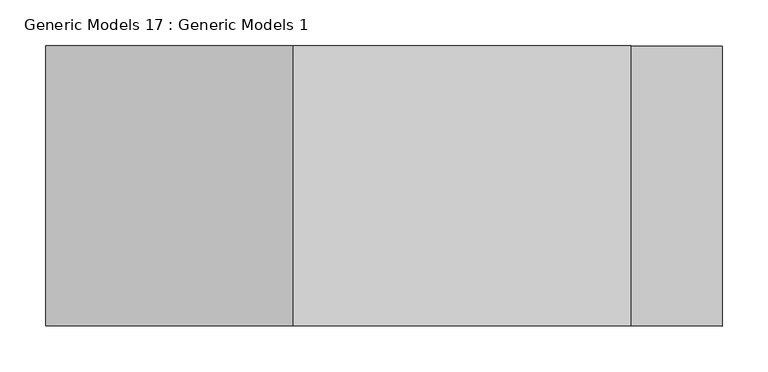
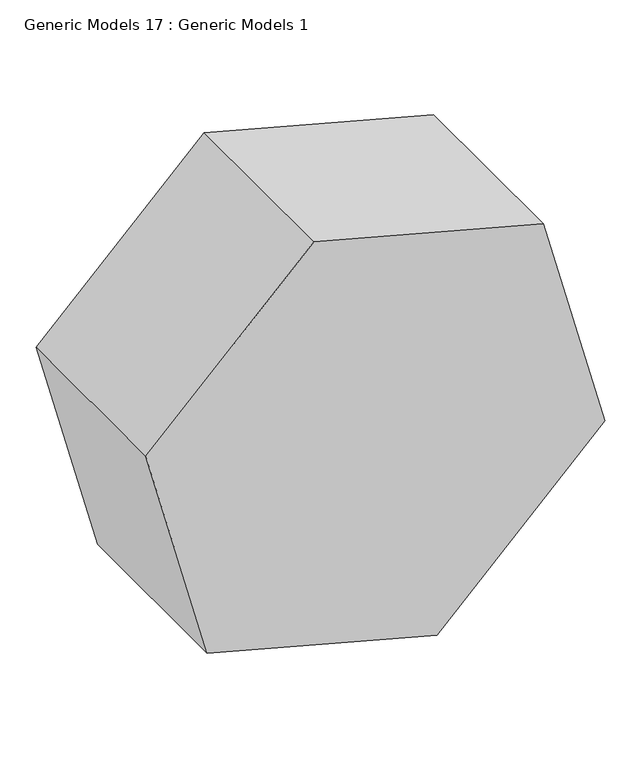
"""IFC4 building model written with IfcOpenShell, lengths in millimetres: proxy geometry, Generic Models 17 : Generic Models 1."""

from ifc_helpers import new_model, si_unit, frame, origin, place, context, project, spatial, polyline, outline, extrude, source, transform, mapped, element, save


def generic_models_17_generic_models_1_fcac293f(model_context):
    return source(origin(), model_context, "Body", "SweptSolid", [
        extrude(outline(polyline([(904.7566299, 7907.4198357), (1003.366686, 7539.4020959), (733.9590024, 7269.9944123), (365.9412626, 7368.6044685), (267.3312064, 7736.6222083), (536.73889, 8006.0298919), (904.7566299, 7907.4198357)])), frame((0.0, -9086.6225464, 0.0), z_axis=(0.0, 1.0, 0.0), x_axis=(0.0, 0.0, 1.0)), (0.0, 0.0, 1.0), 304.8),
    ])


if __name__ == "__main__":
    model = new_model("IFC4")
    model_context = context("Model", 3, world=origin())
    ifc_project = project(units=[si_unit("LENGTHUNIT", "METRE", prefix="MILLI")], contexts=[model_context])
    site = spatial("IfcSite", under=ifc_project)
    building = spatial("IfcBuilding", under=site)
    placement = place(None, origin())
    generic_models_17_generic_models_1_shape = generic_models_17_generic_models_1_fcac293f(model_context)
    element("IfcBuildingElementProxy", 1, Name="Generic Models 17 : Generic Models 1", ObjectType="Generic Models 17 : Generic Models 1", at=placement, inside=building, context=model_context, shape_type="MappedRepresentation", body=[
        mapped(generic_models_17_generic_models_1_shape, transform((0.0, 0.0, 0.0), x_axis=(1.0, 0.0, 0.0), y_axis=(0.0, 1.0, 0.0), z_axis=(0.0, 0.0, 1.0))),
    ])
    save(model, "model.ifc")

# Revit data of these elements
# Element 1 (IfcBuildingElementProxy, "Generic Models 17 : Generic Models 1")
#   Materials on its faces: "Carpet (1)"
# Materials
#   "Carpet (1)": class "Carpet", colour RGB 124 80 67, transparency 0, Description = "Interior finish", Cost = 0
